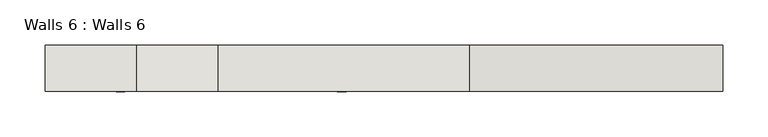
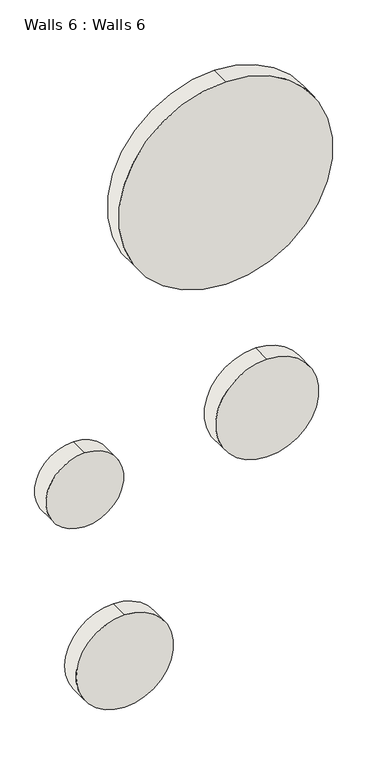
"""IFC4 building model written with IfcOpenShell, lengths in millimetres: wall geometry, Walls 6 : Walls 6."""

from ifc_helpers import new_model, si_unit, point, frame, frame_2d, origin, place, context, project, spatial, circle_curve, trimmed, segment, composite_curve, outline, extrude, source, transform, mapped, element, save


def walls_6_walls_6_dde418cc(model_context):
    return source(origin(), model_context, "Body", "SweptSolid", [
        extrude(outline(composite_curve([segment(trimmed(circle_curve(frame_2d((4718.7007695, -2582.8311901)), 279.4), [point((4439.3007695, -2582.8311901))], [point((4998.1007695, -2582.8311901))], False, "CARTESIAN"), True, "CONTINUOUS"), segment(trimmed(circle_curve(frame_2d((4718.7007695, -2582.8311901)), 279.4), [point((4998.1007695, -2582.8311901))], [point((4439.3007695, -2582.8311901))], False, "CARTESIAN"), True, "CONTINUOUS")], self_intersect=False)), frame((0.0, -4610.7335337, 0.0), z_axis=(0.0, 1.0, 0.0), x_axis=(0.0, 0.0, 1.0)), (0.0, 0.0, 1.0), 50.8137084),
        extrude(outline(composite_curve([segment(trimmed(circle_curve(frame_2d((4001.8954503, -2950.6789272)), 101.6), [point((3900.2954503, -2950.6789272))], [point((4103.4954503, -2950.6789272))], False, "CARTESIAN"), True, "CONTINUOUS"), segment(trimmed(circle_curve(frame_2d((4001.8954503, -2950.6789272)), 101.6), [point((4103.4954503, -2950.6789272))], [point((3900.2954503, -2950.6789272))], False, "CARTESIAN"), True, "CONTINUOUS")], self_intersect=False)), frame((0.0, -4610.7335337, 0.0), z_axis=(0.0, 1.0, 0.0), x_axis=(0.0, 0.0, 1.0)), (0.0, 0.0, 1.0), 50.8137084),
        extrude(outline(composite_curve([segment(trimmed(circle_curve(frame_2d((4060.5259549, -2474.9091512)), 134.7433848), [point((3925.7825701, -2474.9091512))], [point((4195.2693396, -2474.9091512))], False, "CARTESIAN"), True, "CONTINUOUS"), segment(trimmed(circle_curve(frame_2d((4060.5259549, -2474.9091512)), 134.7433848), [point((4195.2693396, -2474.9091512))], [point((3925.7825701, -2474.9091512))], False, "CARTESIAN"), True, "CONTINUOUS")], self_intersect=False)), frame((0.0, -4610.7335337, 0.0), z_axis=(0.0, 1.0, 0.0), x_axis=(0.0, 0.0, 1.0)), (0.0, 0.0, 1.0), 50.8137084),
        extrude(outline(composite_curve([segment(trimmed(circle_curve(frame_2d((3493.6016963, -2846.4006201)), 127.0), [point((3366.6016963, -2846.4006201))], [point((3620.6016963, -2846.4006201))], False, "CARTESIAN"), True, "CONTINUOUS"), segment(trimmed(circle_curve(frame_2d((3493.6016963, -2846.4006201)), 127.0), [point((3620.6016963, -2846.4006201))], [point((3366.6016963, -2846.4006201))], False, "CARTESIAN"), True, "CONTINUOUS")], self_intersect=False)), frame((0.0, -4610.7335337, 0.0), z_axis=(0.0, 1.0, 0.0), x_axis=(0.0, 0.0, 1.0)), (0.0, 0.0, 1.0), 50.8137084),
    ])


if __name__ == "__main__":
    model = new_model("IFC4")
    model_context = context("Model", 3, world=origin())
    ifc_project = project(units=[si_unit("LENGTHUNIT", "METRE", prefix="MILLI")], contexts=[model_context])
    site = spatial("IfcSite", under=ifc_project)
    building = spatial("IfcBuilding", under=site)
    placement = place(None, origin())
    walls_6_walls_6_shape = walls_6_walls_6_dde418cc(model_context)
    element("IfcWall", 1, ObjectType="Walls 6 : Walls 6", at=placement, inside=building, context=model_context, shape_type="MappedRepresentation", body=[
        mapped(walls_6_walls_6_shape, transform((0.0, 0.0, 0.0), x_axis=(1.0, 0.0, 0.0), y_axis=(0.0, 1.0, 0.0), z_axis=(0.0, 0.0, 1.0))),
    ])
    save(model, "model.ifc")

# Revit data of these elements
# Element 1 (IfcWall, "Walls 6 : Walls 6")
#   Materials on its faces: "Default Wall"
# Materials
#   "Default Wall": colour RGB 128 128 128, transparency 0
